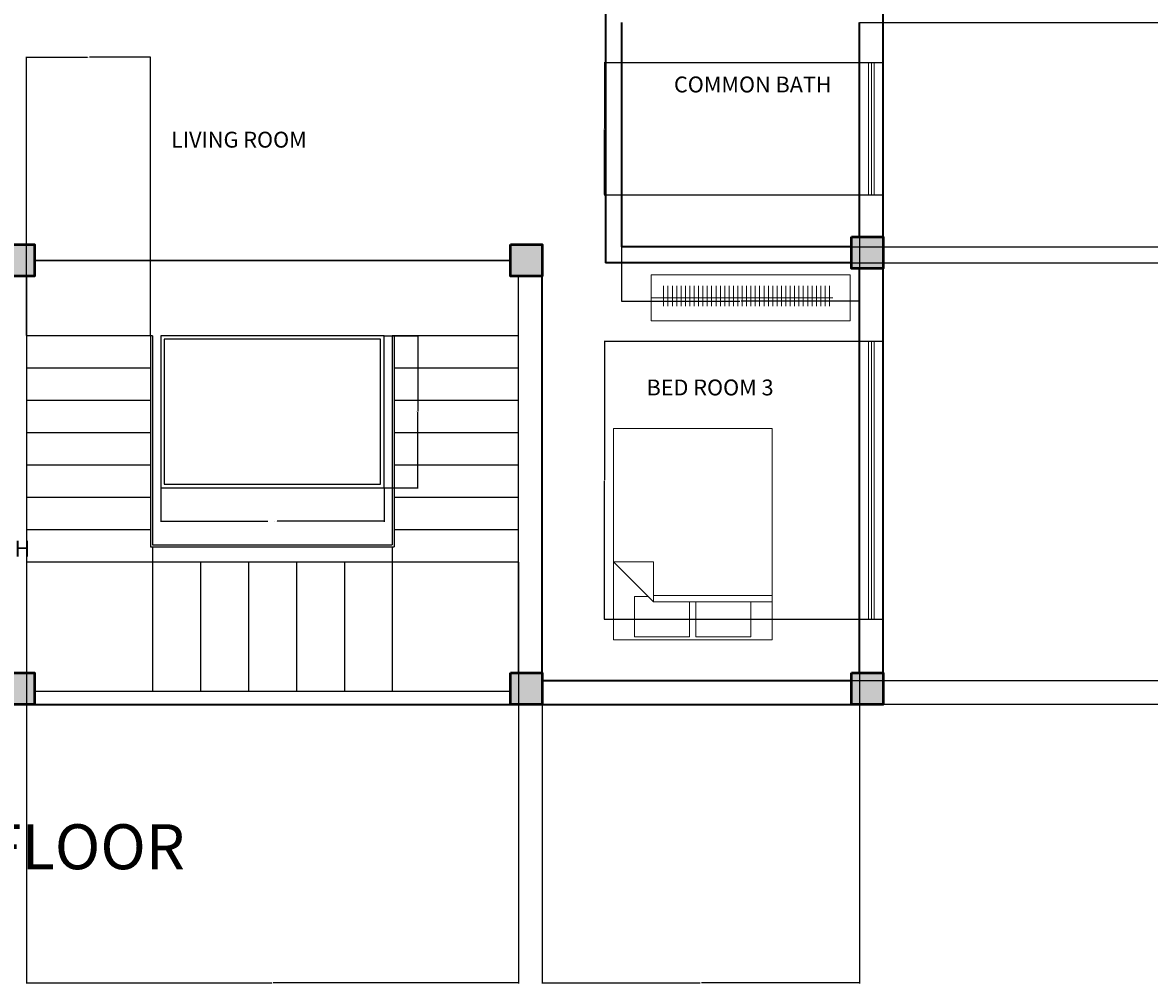
# Model space of a CAD drawing. Units: inches. Extents: x 369 to 4994, y 516 to 1297.
# Tile 2 of 9: x 722 to 1148, y 516 to 880. Entities that reach past the tile are written whole.
import ezdxf

# ---------------------------------------------------------------- set-up
doc = ezdxf.new("R2010")
doc.units = ezdxf.units.IN
doc.header["$MEASUREMENT"] = 0
for name, color, linetype, lineweight in [('A-ANNO-DIMS', 2, 'Continuous', 18), ('A-ANNO-TEXT', 7, 'Continuous', 35), ('A-AREA-IDEN', 7, 'Continuous', 18), ('A-COLS', 7, 'Continuous', 50), ('A-FLOR-CASE', 8, 'Continuous', 18), ('A-FLOR-CASE-PATT', 252, 'Continuous', 13), ('A-FLOR-STRS', 3, 'Continuous', 25), ('A-FURN', 8, 'Continuous', 18), ('A-GLAZ', 4, 'Continuous', 18), ('A-WALL', 7, 'Continuous', 35)]:
    doc.layers.add(name, color=color, linetype=linetype, lineweight=lineweight)
doc.layers.add('A-COLS-PATT', color=18, linetype='Continuous', lineweight=13, true_color=0x000000)
doc.styles.get("Standard").update_dxf_attribs({"font": 'arial.ttf'})
doc.dimstyles.get("Standard").update_dxf_attribs({"dimtxt": 0.18, "dimasz": 0.18, "dimexe": 0.18, "dimexo": 0.0625, "dimgap": 0.09, "dimtad": 0, "dimtih": 1, "dimtoh": 1, "dimdec": 4, "dimzin": 0, "dimdsep": 46, "dimtxsty": 'Standard', "dimcen": 0.09, "dimadec": 0, "dimazin": 0, "dimtfac": 1, "dimtdec": 4, "dimtofl": 0, "dimtmove": 0, "dimatfit": 3, "dimfxl": 1, "dimtolj": 1, "dimtzin": 0, "dimarcsym": 0})

# ---------------------------------------------------------------- blocks, each defined once
blk = doc.blocks.new('Bed - Queen')
for p, q in [((0, -80.00003), (0, 0)), ((0, 0), (59.99999, 0)), ((59.99999, 0), (59.99999, -80.00003)), ((7.99999, -1.2), (28.79998, -1.2)), ((7.99999, -14.4), (7.99999, -1.2)), ((28.79998, -1.2), (28.79998, -14.4)), ((31.19999, -1.2), (51.99999, -1.2)), ((31.19999, -14.4), (31.19999, -1.2)), ((51.99999, -1.2), (51.99999, -16.4)), ((0, -14.4), (44.8, -14.4)), ((44.8, -16.8), (0, -16.8)), ((59.99999, -29.6), (44.8, -14.4)), ((44.8, -14.4), (44.8, -29.6)), ((51.99999, -16.4), (46.79936, -16.4)), ((44.8, -29.6), (59.99999, -29.6)), ((59.99999, -80.00003), (0, -80.00003))]:
    blk.add_line(p, q)
blk = doc.blocks.new('STAIR-WELL-FRAME')
for p, q in [((0, 57.51), (0, 0)), ((84.51, 57.51), (0, 57.51)), ((83.15, 56.15), (1.36, 56.15)), ((1.36, 56.15), (1.36, 1.36)), ((83.15, 1.36), (83.15, 56.15)), ((84.51, 0), (84.51, 57.51)), ((84.51, 0), (84.51, 57.51)), ((1.36, 1.36), (83.15, 1.36)), ((0, 0), (84.51, 0))]:
    blk.add_line(p, q)
blk = doc.blocks.new('*D15')
at = {"layer": 'A-ANNO-DIMS', "color": 0, "lineweight": -2, "transparency": 16777216}
for p, q in [((774, 703.72), (774, 690.92)), ((858.51, 703.72), (858.51, 690.92)), ((774.18, 691.1), (814.51, 691.1)), ((858.33, 691.1), (818.01, 691.1))]:
    blk.add_line(p, q, dxfattribs=at)
at = {"layer": 'A-ANNO-DIMS', "color": 0, "transparency": 16777216}
for points in [[(774.18, 691.13), (774.18, 691.07), (774, 691.1)], [(858.33, 691.13), (858.33, 691.07), (858.51, 691.1)]]:
    blk.add_solid(points, dxfattribs=at)
at = {"layer": 'Defpoints', "color": 0, "transparency": 16777216}
for p in [(774, 703.78), (858.51, 703.78), (858.51, 691.1)]:
    blk.add_point(p, dxfattribs=at)
at = {"layer": 'A-ANNO-DIMS', "color": 0, "transparency": 16777216, "insert": (816.26, 691.1), "char_height": 0.18, "attachment_point": 5}
blk.add_mtext('\\A1;STAIRWELL FRAME 85 TYP.', dxfattribs=at)
blk = doc.blocks.new('*D16')
at = {"layer": 'A-ANNO-DIMS', "color": 0, "lineweight": -2, "transparency": 16777216}
for p, q in [((858.58, 761.29), (871.37, 761.29)), ((871.19, 761.11), (871.19, 732.72)), ((871.19, 703.96), (871.19, 732.36)), ((858.58, 703.78), (871.37, 703.78))]:
    blk.add_line(p, q, dxfattribs=at)
at = {"layer": 'A-ANNO-DIMS', "color": 0, "transparency": 16777216}
for points in [[(871.16, 761.11), (871.22, 761.11), (871.19, 761.29)], [(871.16, 703.96), (871.22, 703.96), (871.19, 703.78)]]:
    blk.add_solid(points, dxfattribs=at)
at = {"layer": 'Defpoints', "color": 0, "transparency": 16777216}
for p in [(858.51, 761.29), (871.19, 761.29), (858.51, 703.78)]:
    blk.add_point(p, dxfattribs=at)
at = {"layer": 'A-ANNO-DIMS', "color": 0, "transparency": 16777216, "insert": (871.19, 732.54), "char_height": 0.18, "attachment_point": 5}
blk.add_mtext('\\A1;58 TYP.', dxfattribs=at)
blk = doc.blocks.new('*D47')
at = {"layer": 'A-ANNO-DIMS', "color": 0, "lineweight": -2, "transparency": 16777216}
for p, q in [((1038.32, 879.79), (2671.51, 879.79)), ((2671.33, 879.61), (2671.33, 837.52)), ((2671.33, 795.07), (2671.33, 837.16)), ((1035.32, 794.89), (2671.51, 794.89))]:
    blk.add_line(p, q, dxfattribs=at)
at = {"layer": 'A-ANNO-DIMS', "color": 0, "transparency": 16777216}
for points in [[(2671.3, 879.61), (2671.36, 879.61), (2671.33, 879.79)], [(2671.3, 795.07), (2671.36, 795.07), (2671.33, 794.89)]]:
    blk.add_solid(points, dxfattribs=at)
at = {"layer": 'Defpoints', "color": 0, "transparency": 16777216}
for p in [(1038.26, 879.79), (2671.33, 879.79), (1035.26, 794.89)]:
    blk.add_point(p, dxfattribs=at)
at = {"layer": 'A-ANNO-DIMS', "color": 0, "transparency": 16777216, "insert": (2671.33, 837.34), "char_height": 0.18, "attachment_point": 5}
blk.add_mtext('\\A1;84.9', dxfattribs=at)
blk = doc.blocks.new('*D50')
at = {"layer": 'A-ANNO-DIMS', "color": 0, "lineweight": -2, "transparency": 16777216}
for p, q in [((723.26, 675.6), (723.26, 516.21)), ((909.26, 675.6), (909.26, 516.21)), ((723.44, 516.39), (815.98, 516.39)), ((909.08, 516.39), (816.54, 516.39))]:
    blk.add_line(p, q, dxfattribs=at)
at = {"layer": 'A-ANNO-DIMS', "color": 0, "transparency": 16777216}
for points in [[(723.44, 516.42), (723.44, 516.36), (723.26, 516.39)], [(909.08, 516.42), (909.08, 516.36), (909.26, 516.39)]]:
    blk.add_solid(points, dxfattribs=at)
at = {"layer": 'Defpoints', "color": 0, "transparency": 16777216}
for p in [(723.26, 675.66), (909.26, 675.66), (909.26, 516.39)]:
    blk.add_point(p, dxfattribs=at)
at = {"layer": 'A-ANNO-DIMS', "color": 0, "transparency": 16777216, "insert": (816.26, 516.39), "char_height": 0.18, "attachment_point": 5}
blk.add_mtext('\\A1;186', dxfattribs=at)
blk = doc.blocks.new('*D51')
at = {"layer": 'A-ANNO-DIMS', "color": 0, "lineweight": -2, "transparency": 16777216}
for p, q in [((1038.26, 633.73), (1038.26, 516.21)), ((918.26, 630.73), (918.26, 516.21)), ((918.44, 516.39), (977.98, 516.39)), ((1038.08, 516.39), (978.54, 516.39))]:
    blk.add_line(p, q, dxfattribs=at)
at = {"layer": 'A-ANNO-DIMS', "color": 0, "transparency": 16777216}
for points in [[(918.44, 516.42), (918.44, 516.36), (918.26, 516.39)], [(1038.08, 516.42), (1038.08, 516.36), (1038.26, 516.39)]]:
    blk.add_solid(points, dxfattribs=at)
at = {"layer": 'Defpoints', "color": 0, "transparency": 16777216}
for p in [(918.26, 630.79), (1038.26, 633.79), (1038.26, 516.39)]:
    blk.add_point(p, dxfattribs=at)
at = {"layer": 'A-ANNO-DIMS', "color": 0, "transparency": 16777216, "insert": (978.26, 516.39), "char_height": 0.18, "attachment_point": 5}
blk.add_mtext('\\A1;120', dxfattribs=at)
blk = doc.blocks.new('*D52')
at = {"layer": 'A-ANNO-DIMS', "color": 0, "lineweight": -2, "transparency": 16777216}
for p, q in [((942.32, 788.89), (2671.51, 788.89)), ((2671.33, 788.71), (2671.33, 710.02)), ((2671.33, 630.97), (2671.33, 709.66)), ((1035.32, 630.79), (2671.51, 630.79))]:
    blk.add_line(p, q, dxfattribs=at)
at = {"layer": 'A-ANNO-DIMS', "color": 0, "transparency": 16777216}
for points in [[(2671.3, 788.71), (2671.36, 788.71), (2671.33, 788.89)], [(2671.3, 630.97), (2671.36, 630.97), (2671.33, 630.79)]]:
    blk.add_solid(points, dxfattribs=at)
at = {"layer": 'Defpoints', "color": 0, "transparency": 16777216}
for p in [(942.26, 788.89), (2671.33, 788.89), (1035.26, 630.79)]:
    blk.add_point(p, dxfattribs=at)
at = {"layer": 'A-ANNO-DIMS', "color": 0, "transparency": 16777216, "insert": (2671.33, 709.84), "char_height": 0.18, "attachment_point": 5}
blk.add_mtext('\\A1;158.1', dxfattribs=at)
blk = doc.blocks.new('*D55')
at = {"layer": 'A-ANNO-DIMS', "color": 0, "lineweight": -2, "transparency": 16777216}
for p, q in [((948.26, 879.73), (948.26, 774.21)), ((1038.26, 879.73), (1038.26, 774.21)), ((948.44, 774.39), (993.04, 774.39)), ((1038.08, 774.39), (993.48, 774.39))]:
    blk.add_line(p, q, dxfattribs=at)
at = {"layer": 'A-ANNO-DIMS', "color": 0, "transparency": 16777216}
for points in [[(948.44, 774.42), (948.44, 774.36), (948.26, 774.39)], [(1038.08, 774.42), (1038.08, 774.36), (1038.26, 774.39)]]:
    blk.add_solid(points, dxfattribs=at)
at = {"layer": 'Defpoints', "color": 0, "transparency": 16777216}
for p in [(948.26, 879.79), (1038.26, 879.79), (948.26, 774.39)]:
    blk.add_point(p, dxfattribs=at)
at = {"layer": 'A-ANNO-DIMS', "color": 0, "transparency": 16777216, "insert": (993.26, 774.39), "char_height": 0.18, "attachment_point": 5}
blk.add_mtext('\\A1;90', dxfattribs=at)
blk = doc.blocks.new('*D66')
at = {"layer": 'A-ANNO-DIMS', "color": 0, "lineweight": -2, "transparency": 16777216}
for p, q in [((1047.2, 864.56), (941.68, 864.56)), ((941.86, 864.38), (941.86, 839.72)), ((941.86, 814.71), (941.86, 839.36)), ((1047.2, 814.53), (941.68, 814.53))]:
    blk.add_line(p, q, dxfattribs=at)
at = {"layer": 'A-ANNO-DIMS', "color": 0, "transparency": 16777216}
for points in [[(941.83, 864.38), (941.89, 864.38), (941.86, 864.56)], [(941.83, 814.71), (941.89, 814.71), (941.86, 814.53)]]:
    blk.add_solid(points, dxfattribs=at)
at = {"layer": 'Defpoints', "color": 0, "transparency": 16777216}
for p in [(941.86, 864.56), (1047.26, 864.56), (1047.26, 814.53)]:
    blk.add_point(p, dxfattribs=at)
at = {"layer": 'A-ANNO-DIMS', "color": 0, "transparency": 16777216, "insert": (941.86, 839.54), "char_height": 0.18, "attachment_point": 5}
blk.add_mtext('\\A1;50.03', dxfattribs=at)
blk = doc.blocks.new('*D67')
at = {"layer": 'A-ANNO-DIMS', "color": 0, "lineweight": -2, "transparency": 16777216}
for p, q in [((1047.2, 759.14), (941.68, 759.14)), ((941.86, 758.96), (941.86, 706.7)), ((941.86, 654.08), (941.86, 706.33)), ((1047.2, 653.9), (941.68, 653.9))]:
    blk.add_line(p, q, dxfattribs=at)
at = {"layer": 'A-ANNO-DIMS', "color": 0, "transparency": 16777216}
for points in [[(941.83, 758.96), (941.89, 758.96), (941.86, 759.14)], [(941.83, 654.08), (941.89, 654.08), (941.86, 653.9)]]:
    blk.add_solid(points, dxfattribs=at)
at = {"layer": 'Defpoints', "color": 0, "transparency": 16777216}
for p in [(941.86, 759.14), (1047.26, 759.14), (1047.26, 653.9)]:
    blk.add_point(p, dxfattribs=at)
at = {"layer": 'A-ANNO-DIMS', "color": 0, "transparency": 16777216, "insert": (941.86, 706.52), "char_height": 0.18, "attachment_point": 5}
blk.add_mtext('\\A1;105.24', dxfattribs=at)
blk = doc.blocks.new('*D73')
at = {"layer": 'A-ANNO-DIMS', "color": 0, "lineweight": -2, "transparency": 16777216}
for p, q in [((723.26, 761.36), (723.26, 866.87)), ((723.44, 866.69), (746.33, 866.69)), ((770.03, 866.69), (747.13, 866.69)), ((770.21, 761.36), (770.21, 866.87))]:
    blk.add_line(p, q, dxfattribs=at)
at = {"layer": 'A-ANNO-DIMS', "color": 0, "transparency": 16777216}
for points in [[(723.44, 866.72), (723.44, 866.66), (723.26, 866.69)], [(770.03, 866.72), (770.03, 866.66), (770.21, 866.69)]]:
    blk.add_solid(points, dxfattribs=at)
at = {"layer": 'Defpoints', "color": 0, "transparency": 16777216}
for p in [(770.21, 866.69), (723.26, 761.29), (770.21, 761.29)]:
    blk.add_point(p, dxfattribs=at)
at = {"layer": 'A-ANNO-DIMS', "color": 0, "transparency": 16777216, "insert": (746.73, 866.69), "char_height": 0.18, "attachment_point": 5}
blk.add_mtext('\\A1;46.95', dxfattribs=at)
blk = doc.blocks.new('*D75')
at = {"layer": 'A-ANNO-DIMS', "color": 0, "lineweight": -2, "transparency": 16777216}
for p, q in [((1208.31, 1038.79), (368.68, 1038.79)), ((368.86, 1038.61), (368.86, 830.47)), ((368.86, 621.97), (368.86, 830.11)), ((1262.31, 621.79), (368.68, 621.79))]:
    blk.add_line(p, q, dxfattribs=at)
at = {"layer": 'A-ANNO-DIMS', "color": 0, "transparency": 16777216}
for points in [[(368.83, 1038.61), (368.89, 1038.61), (368.86, 1038.79)], [(368.83, 621.97), (368.89, 621.97), (368.86, 621.79)]]:
    blk.add_solid(points, dxfattribs=at)
at = {"layer": 'Defpoints', "color": 0, "transparency": 16777216}
for p in [(368.86, 1038.79), (1208.37, 1038.79), (1262.37, 621.79)]:
    blk.add_point(p, dxfattribs=at)
at = {"layer": 'A-ANNO-DIMS', "color": 0, "transparency": 16777216, "insert": (368.86, 830.29), "char_height": 0.18, "attachment_point": 5}
blk.add_mtext('\\A1;417', dxfattribs=at)
blk = doc.blocks.new('*D98')
at = {"layer": 'A-ANNO-DIMS', "color": 0, "lineweight": -2, "transparency": 16777216}
for p, q in [((1992.86, 1038.79), (368.68, 1038.79)), ((368.86, 1038.61), (368.86, 830.47)), ((368.86, 621.97), (368.86, 830.11)), ((2046.86, 621.79), (368.68, 621.79))]:
    blk.add_line(p, q, dxfattribs=at)
at = {"layer": 'A-ANNO-DIMS', "color": 0, "transparency": 16777216}
for points in [[(368.83, 1038.61), (368.89, 1038.61), (368.86, 1038.79)], [(368.83, 621.97), (368.89, 621.97), (368.86, 621.79)]]:
    blk.add_solid(points, dxfattribs=at)
at = {"layer": 'Defpoints', "color": 0, "transparency": 16777216}
for p in [(368.86, 1038.79), (1992.93, 1038.79), (2046.93, 621.79)]:
    blk.add_point(p, dxfattribs=at)
at = {"layer": 'A-ANNO-DIMS', "color": 0, "transparency": 16777216, "insert": (368.86, 830.29), "char_height": 0.18, "attachment_point": 5}
blk.add_mtext('\\A1;417', dxfattribs=at)

msp = doc.modelspace()

# ---------------------------------------------------------------- hatches: boundary and pattern name
at = {"layer": 'A-COLS-PATT'}
h = msp.add_hatch(color=256, dxfattribs=at)
h.dxf.hatch_style = 1
h.paths.add_polyline_path([(540.2581, 633.7894), (528.2581, 633.7894), (528.2581, 621.7894), (540.2581, 621.7894)])
h.paths.add_polyline_path([(726.2581, 633.7894), (714.2581, 633.7894), (714.2581, 621.7894), (726.2581, 621.7894)])
h.paths.add_polyline_path([(918.2581, 633.7894), (906.2581, 633.7894), (906.2581, 621.7894), (918.2581, 621.7894)])
h.paths.add_polyline_path([(1047.2581, 633.7894), (1035.2581, 633.7894), (1035.2581, 621.7894), (1047.2581, 621.7894)])
h.paths.add_polyline_path([(1047.2581, 798.6977), (1035.2581, 798.6977), (1035.2581, 786.6977), (1047.2581, 786.6977)])
h.paths.add_polyline_path([(918.2581, 795.7894), (906.2581, 795.7894), (906.2581, 783.7894), (918.2581, 783.7894)])
h.paths.add_polyline_path([(726.2581, 795.7894), (714.2581, 795.7894), (714.2581, 783.7894), (726.2581, 783.7894)])
h.paths.add_polyline_path([(1047.2581, 1038.7894), (1035.2581, 1038.7894), (1035.2581, 1026.7894), (1047.2581, 1026.7894)])
h.paths.add_polyline_path([(855.044, 1038.7894), (843.044, 1038.7894), (843.044, 1026.7894), (855.044, 1026.7894)])
h.paths.add_polyline_path([(728.5536, 1038.7894), (716.5536, 1038.7894), (716.5536, 1026.7894), (728.5536, 1026.7894)])
h.paths.add_polyline_path([(543.2581, 1038.7894), (531.2581, 1038.7894), (531.2581, 1026.7894), (543.2581, 1026.7894)])
h.paths.add_polyline_path([(543.2581, 792.9013), (531.2581, 792.9013), (531.2581, 780.9013), (543.2581, 780.9013), (543.2581, 783.7894)])
h.paths.add_polyline_path([(1274.3738, 633.7894), (1262.3738, 633.7894), (1262.3738, 621.7894), (1274.3738, 621.7894)])
h.paths.add_polyline_path([(1460.3738, 633.7894), (1448.3738, 633.7894), (1448.3738, 621.7894), (1460.3738, 621.7894)])
h.paths.add_polyline_path([(1652.3738, 633.7894), (1640.3738, 633.7894), (1640.3738, 621.7894), (1652.3738, 621.7894)])
h.paths.add_polyline_path([(1781.3738, 633.7894), (1769.3738, 633.7894), (1769.3738, 621.7894), (1781.3738, 621.7894)])
h.paths.add_polyline_path([(1781.3738, 1038.7894), (1769.3738, 1038.7894), (1769.3738, 1026.7894), (1781.3738, 1026.7894)])
h.paths.add_polyline_path([(1625.484, 1038.7894), (1613.484, 1038.7894), (1613.484, 1026.7894), (1615.6962, 1026.7894), (1625.484, 1026.7894)])
h.paths.add_polyline_path([(1462.6692, 1038.7894), (1450.6692, 1038.7894), (1450.6692, 1026.7894), (1462.6692, 1026.7894)])
h.paths.add_polyline_path([(1277.3738, 1038.7894), (1265.3738, 1038.7894), (1265.3738, 1026.7894), (1277.3738, 1026.7894)])
h.paths.add_polyline_path([(1460.3738, 807.7894), (1448.3738, 807.7894), (1448.3738, 795.7894), (1460.3738, 795.7894)])
h.paths.add_polyline_path([(1652.3738, 807.7894), (1640.3738, 807.7894), (1640.3738, 795.7894), (1652.3738, 795.7894)])
h.paths.add_polyline_path([(2244.9265, 633.7894), (2232.9265, 633.7894), (2232.9265, 621.7894), (2244.9265, 621.7894)])
h.paths.add_polyline_path([(2058.9265, 633.7894), (2046.9265, 633.7894), (2046.9265, 621.7894), (2058.9265, 621.7894)])
h.paths.add_polyline_path([(2436.9265, 633.7894), (2424.9265, 633.7894), (2424.9265, 621.7894), (2436.9265, 621.7894)])
h.paths.add_polyline_path([(2565.9265, 633.7894), (2553.9265, 633.7894), (2553.9265, 621.7894), (2565.9265, 621.7894)])
h.paths.add_polyline_path([(2565.9265, 798.6977), (2553.9265, 798.6977), (2553.9265, 786.6977), (2565.9265, 786.6977)])
h.paths.add_polyline_path([(2565.9265, 1038.7894), (2553.9265, 1038.7894), (2553.9265, 1026.7894), (2565.9265, 1026.7894)])
h.paths.add_polyline_path([(2436.9265, 1038.7894), (2424.9265, 1038.7894), (2424.9265, 1026.7894), (2436.9265, 1026.7894)])
h.paths.add_polyline_path([(2247.222, 1038.7894), (2235.222, 1038.7894), (2235.222, 1026.7894), (2247.222, 1026.7894)])
h.paths.add_polyline_path([(2061.9265, 1038.7894), (2049.9265, 1038.7894), (2049.9265, 1026.7894), (2061.9265, 1026.7894)])
at = {"layer": 'A-FLOR-CASE-PATT'}
h = msp.add_hatch(dxfattribs=at)
h.set_pattern_fill('ANSI31', color=256, scale=13.2082, angle=45, style=0)
h.paths.add_polyline_path([(963.2915, 772.411), (1027.6415, 772.411), (1027.6415, 780.181), (963.2915, 780.181)])

# ---------------------------------------------------------------- linework, layer by layer
at = {"layer": 'A-COLS'}
for points in [[(1035.2581, 798.6977), (1047.2581, 798.6977), (1047.2581, 786.6977), (1035.2581, 786.6977)], [(714.2581, 795.7894), (726.2581, 795.7894), (726.2581, 783.7894), (714.2581, 783.7894)], [(906.2581, 795.7894), (918.2581, 795.7894), (918.2581, 783.7894), (906.2581, 783.7894)], [(906.2581, 633.7894), (918.2581, 633.7894), (918.2581, 621.7894), (906.2581, 621.7894)], [(1035.2581, 633.7894), (1047.2581, 633.7894), (1047.2581, 621.7894), (1035.2581, 621.7894)]]:
    msp.add_lwpolyline(points, close=True, dxfattribs=at)
msp.add_lwpolyline([(726.2581, 621.7894), (714.2581, 621.7894), (714.2581, 633.7894), (726.2581, 633.7894), (726.2581, 621.7894)], dxfattribs=at)
at = {"layer": 'A-FLOR-CASE'}
msp.add_line((959.4718, 775.5948), (1028.2003, 775.5948), dxfattribs=at)
msp.add_lwpolyline([(959.4718, 766.8842), (959.4718, 784.3054), (1034.7279, 784.3054), (1034.7279, 766.8842)], close=True, dxfattribs=at)
at = {"layer": 'A-FLOR-STRS'}
for p, q in [((726.2581, 795.7894), (714.2581, 795.7894)), ((726.2581, 789.7894), (906.2581, 789.7894)), ((906.2581, 789.7894), (726.2581, 789.7894)), ((723.2581, 783.7894), (723.2581, 765.7894)), ((909.2581, 633.7894), (909.2581, 783.7894)), ((723.2581, 765.7894), (723.2581, 633.7894)), ((770.9222, 761.2935), (723.2581, 761.2935)), ((770.2064, 761.2935), (770.2064, 681.4595)), ((770.9222, 761.2935), (770.9222, 682.1754)), ((909.2581, 761.2935), (861.5941, 761.2935)), ((861.5941, 761.2935), (861.5941, 682.1754)), ((862.3099, 761.2935), (862.3099, 681.4595)), ((770.2064, 749.0604), (723.2581, 749.0604)), ((909.2581, 749.0604), (862.3099, 749.0604)), ((770.2064, 736.8273), (723.2581, 736.8273)), ((909.2581, 736.8273), (862.3099, 736.8273)), ((770.2064, 724.5942), (723.2581, 724.5942)), ((909.2581, 724.5942), (862.3099, 724.5942)), ((770.2064, 712.361), (723.2581, 712.361)), ((909.2581, 712.361), (862.3099, 712.361)), ((770.2064, 700.1279), (723.2581, 700.1279)), ((909.2581, 700.1279), (862.3099, 700.1279)), ((770.2064, 687.8948), (723.2581, 687.8948)), ((909.2581, 687.8948), (862.3099, 687.8948)), ((770.9222, 682.1754), (861.5941, 682.1754)), ((770.2064, 681.4595), (862.3099, 681.4595)), ((770.9222, 681.4595), (770.9222, 626.7293)), ((861.5941, 681.4595), (861.5941, 626.7293)), ((909.2581, 675.6617), (723.2581, 675.6617)), ((789.0566, 675.6617), (789.0566, 626.7293)), ((807.191, 675.6617), (807.191, 626.7293)), ((825.3253, 675.6617), (825.3253, 626.7293)), ((843.4597, 675.6617), (843.4597, 626.7293)), ((861.5941, 675.6617), (861.5941, 626.7293)), ((906.2581, 626.7293), (726.2581, 626.7293))]:
    msp.add_line(p, q, dxfattribs=at)
at = {"layer": 'A-GLAZ'}
for p, q in [((1041.6821, 814.5265), (1041.6821, 864.5582)), ((1042.7581, 814.5265), (1042.7581, 864.5582)), ((1043.8342, 814.5265), (1043.8342, 864.5582)), ((1041.6821, 653.8974), (1041.6821, 759.1364)), ((1041.6821, 653.8974), (1041.6821, 759.1364)), ((1042.7581, 653.8974), (1042.7581, 759.1364)), ((1043.8342, 653.8974), (1043.8342, 759.1364))]:
    msp.add_line(p, q, dxfattribs=at)
for points in [[(1047.2581, 814.5265), (1038.2581, 814.5265), (1038.2581, 864.5582), (1047.2581, 864.5582)], [(1047.2581, 653.8974), (1038.2581, 653.8974), (1038.2581, 759.1364), (1047.2581, 759.1364)]]:
    msp.add_lwpolyline(points, close=True, dxfattribs=at)
at = {"layer": 'A-WALL'}
for p, q in [((1047.2581, 621.7894), (1047.2581, 1029.7894)), ((942.2581, 885.7894), (942.2581, 788.8925)), ((948.2581, 879.7894), (948.2581, 794.8925)), ((1038.2581, 798.6977), (1038.2581, 879.7894)), ((918.2581, 795.7894), (906.2581, 795.7894)), ((918.2581, 621.7894), (918.2581, 795.7894)), ((1035.2581, 794.8925), (948.2581, 794.8925)), ((1035.2581, 788.8925), (942.2581, 788.8925)), ((1038.2581, 633.7894), (1038.2581, 786.6977)), ((1038.2581, 771.7894), (1038.2581, 786.6977)), ((918.2581, 630.7894), (1035.2581, 630.7894)), ((726.2581, 621.7894), (918.2581, 621.7894)), ((918.2581, 621.7894), (1047.2581, 621.7894))]:
    msp.add_line(p, q, dxfattribs=at)

# ---------------------------------------------------------------- block references
at = {"layer": 'A-FLOR-STRS'}
msp.add_blockref('STAIR-WELL-FRAME', (774.002, 703.781), dxfattribs=at)
at = {"layer": 'A-FURN', "rotation": 180}
msp.add_blockref('Bed - Queen', (1005.2308, 646.1814), dxfattribs=at)

# ---------------------------------------------------------------- texts
at = {"layer": 'A-ANNO-TEXT'}
msp.add_text('GROUND FLOOR ', height=17.017766, dxfattribs=at).set_placement((605.8748, 559.4225))
at = {"layer": 'A-AREA-IDEN'}
for s, p in [('COMMON BATH', (968.1112, 853.3527)), ('LIVING ROOM ', (777.9021, 832.4687)), ('BED ROOM 3', (957.7565, 738.713)), ('COMMAN BATH ', (666.1342, 677.737))]:
    msp.add_text(s, height=6, dxfattribs=at).set_placement(p)

# ---------------------------------------------------------------- dimensions: what is measured, and where the dimension line sits
at = {"layer": 'A-ANNO-DIMS'}
for base, p1, p2, angle, override, picture, middle in [((368.8581, 1038.7894), (1262.3738, 621.7894), (1208.3738, 1038.7894), 90, {"dimdec": 0, "dimlfac": 1, "dimrnd": 0, "dimzin": 0, "dimdsep": 46, "dimlunit": 2}, '*D75', (368.8581, 830.2894)), ((368.8581, 1038.7894), (2046.9265, 621.7894), (1992.9265, 1038.7894), 90, {"dimdec": 0, "dimlfac": 1, "dimrnd": 0, "dimzin": 0, "dimdsep": 46, "dimlunit": 2}, '*D98', (368.8581, 830.2894)), ((948.2581, 774.3894), (1038.2581, 879.7894), (948.2581, 879.7894), 180, {"dimdec": 0, "dimlfac": 1, "dimrnd": 0, "dimzin": 0, "dimdsep": 46, "dimlunit": 2}, '*D55', (993.2581, 774.3894)), ((2671.3265, 879.7894), (1035.2581, 794.8925), (1038.2581, 879.7894), 90, {"dimdec": 1, "dimlfac": 1, "dimrnd": 0, "dimzin": 0, "dimdsep": 46, "dimlunit": 2}, '*D47', (2671.3265, 837.3409)), ((770.2064, 866.6935), (723.2581, 761.2935), (770.2064, 761.2935), 0, {"dimdec": 2, "dimlfac": 1, "dimrnd": 0, "dimzin": 0, "dimdsep": 46, "dimlunit": 2}, '*D73', (746.7322, 866.6935)), ((941.8581, 864.5582), (1047.2581, 814.5265), (1047.2581, 864.5582), 90, {"dimdec": 2, "dimlfac": 1, "dimrnd": 0, "dimzin": 0, "dimdsep": 46, "dimlunit": 2}, '*D66', (941.8581, 839.5424)), ((2671.3265, 788.8925), (1035.2581, 630.7894), (942.2581, 788.8925), 90, {"dimdec": 1, "dimlfac": 1, "dimrnd": 0, "dimzin": 0, "dimdsep": 46, "dimlunit": 2}, '*D52', (2671.3265, 709.8409)), ((941.8581, 759.1364), (1047.2581, 653.8974), (1047.2581, 759.1364), 90, {"dimdec": 2, "dimlfac": 1, "dimrnd": 0, "dimzin": 0, "dimdsep": 46, "dimlunit": 2}, '*D67', (941.8581, 706.5169))]:
    dim = msp.add_linear_dim(base=base, p1=p1, p2=p2, angle=angle, dimstyle='Standard', override=override, dxfattribs=at)
    dim.commit()
    dim.dimension.update_dxf_attribs({"geometry": picture, "text_midpoint": middle})
dim = msp.add_linear_dim(base=(871.1915, 761.2935), p1=(858.5146, 703.7806), p2=(858.5146, 761.2935), angle=90, text='<> TYP.', dimstyle='Standard', override={"dimdec": 0, "dimlfac": 1, "dimrnd": 0, "dimzin": 0, "dimdsep": 46, "dimlunit": 2}, dxfattribs=at)
dim.commit()
dim.dimension.update_dxf_attribs({"geometry": '*D16', "text_midpoint": (871.1915, 732.537)})
dim = msp.add_linear_dim(base=(858.5146, 691.1037), p1=(774.0017, 703.7806), p2=(858.5146, 703.7806), text='STAIRWELL FRAME <> TYP.', dimstyle='Standard', override={"dimdec": 0, "dimlfac": 1, "dimrnd": 0, "dimzin": 0, "dimdsep": 46, "dimlunit": 2}, dxfattribs=at)
dim.commit()
dim.dimension.update_dxf_attribs({"geometry": '*D15', "text_midpoint": (816.2581, 691.1037)})
for base, p1, p2, picture, middle in [((909.2581, 516.3894), (723.2581, 675.6617), (909.2581, 675.6617), '*D50', (816.2581, 516.3894)), ((1038.2581, 516.3894), (918.2581, 630.7894), (1038.2581, 633.7894), '*D51', (978.2581, 516.3894))]:
    dim = msp.add_linear_dim(base=base, p1=p1, p2=p2, dimstyle='Standard', override={"dimdec": 0, "dimlfac": 1, "dimrnd": 0, "dimzin": 0, "dimdsep": 46, "dimlunit": 2}, dxfattribs=at)
    dim.commit()
    dim.dimension.update_dxf_attribs({"geometry": picture, "text_midpoint": middle})

doc.saveas('drawing.dxf')
